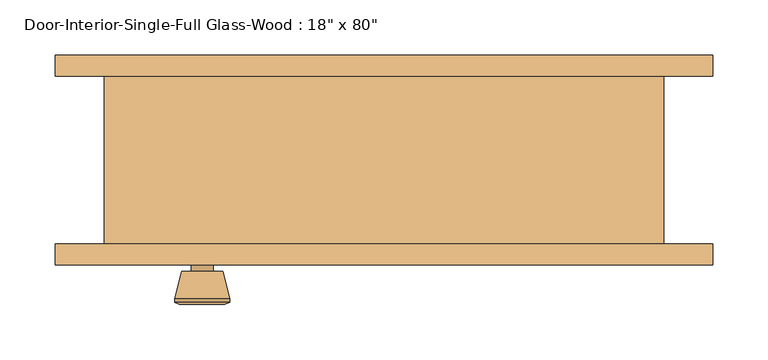
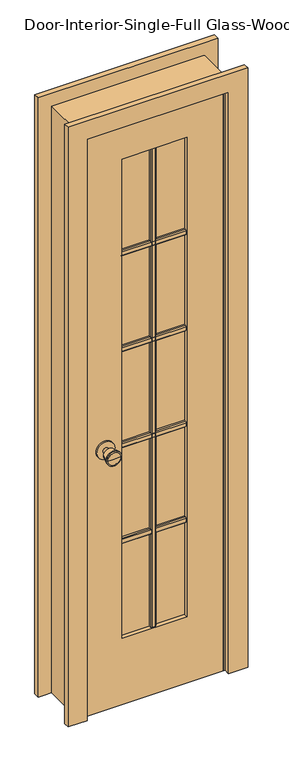
"""IFC4 building model written with IfcOpenShell, lengths in millimetres: door geometry."""

from ifc_helpers import new_model, si_unit, point, frame, frame_2d, origin, place, context, project, spatial, polyline, circle_curve, trimmed, segment, composite_curve, outline, extrude, faceted_brep, source, transform, mapped, element, save
from ifc_brep_helpers import plane_surface, cylinder_surface, revolved_surface, advanced_brep


def door_059bf842(model_context):
    return source(origin(), model_context, "Body", "SolidModel", [
        extrude(outline(polyline([(-59.055, 1586.23), (-59.055, 1567.18), (-65.405, 1567.18), (-68.58, 1570.355), (-68.58, 1583.055), (-65.405, 1586.23), (-59.055, 1586.23)])), frame((-107.95, 0.0, 0.0), z_axis=(1.0, 0.0, 0.0), x_axis=(0.0, 1.0, 0.0)), (0.0, 0.0, 1.0), 215.9),
        extrude(outline(polyline([(-59.055, 1249.9975), (-59.055, 1230.9475), (-65.405, 1230.9475), (-68.58, 1234.1225), (-68.58, 1246.8225), (-65.405, 1249.9975), (-59.055, 1249.9975)])), frame((-107.95, 0.0, 0.0), z_axis=(1.0, 0.0, 0.0), x_axis=(0.0, 1.0, 0.0)), (0.0, 0.0, 1.0), 215.9),
        extrude(outline(polyline([(-59.055, 913.765), (-59.055, 894.715), (-65.405, 894.715), (-68.58, 897.89), (-68.58, 910.59), (-65.405, 913.765), (-59.055, 913.765)])), frame((-107.95, 0.0, 0.0), z_axis=(1.0, 0.0, 0.0), x_axis=(0.0, 1.0, 0.0)), (0.0, 0.0, 1.0), 215.9),
        extrude(outline(polyline([(-9.525, -59.055), (9.525, -59.055), (9.525, -65.405), (6.35, -68.58), (-6.35, -68.58), (-9.525, -65.405), (-9.525, -59.055)])), frame((0.0, 0.0, 231.775), z_axis=(0.0, 0.0, 1.0), x_axis=(1.0, 0.0, 0.0)), (0.0, 0.0, 1.0), 1681.1625),
        extrude(outline(polyline([(-59.055, 577.5325), (-59.055, 558.4825), (-65.405, 558.4825), (-68.58, 561.6575), (-68.58, 574.3575), (-65.405, 577.5325), (-59.055, 577.5325)])), frame((-107.95, 0.0, 0.0), z_axis=(1.0, 0.0, 0.0), x_axis=(0.0, 1.0, 0.0)), (0.0, 0.0, 1.0), 215.9),
        extrude(outline(polyline([(-52.07, 1586.23), (-45.72, 1586.23), (-42.545, 1583.055), (-42.545, 1570.355), (-45.72, 1567.18), (-52.07, 1567.18), (-52.07, 1586.23)])), frame((-107.95, 0.0, 0.0), z_axis=(1.0, 0.0, 0.0), x_axis=(0.0, 1.0, 0.0)), (0.0, 0.0, 1.0), 215.9),
        extrude(outline(polyline([(-52.07, 1249.9975), (-45.72, 1249.9975), (-42.545, 1246.8225), (-42.545, 1234.1225), (-45.72, 1230.9475), (-52.07, 1230.9475), (-52.07, 1249.9975)])), frame((-107.95, 0.0, 0.0), z_axis=(1.0, 0.0, 0.0), x_axis=(0.0, 1.0, 0.0)), (0.0, 0.0, 1.0), 215.9),
        extrude(outline(polyline([(-52.07, 913.765), (-45.72, 913.765), (-42.545, 910.59), (-42.545, 897.89), (-45.72, 894.715), (-52.07, 894.715), (-52.07, 913.765)])), frame((-107.95, 0.0, 0.0), z_axis=(1.0, 0.0, 0.0), x_axis=(0.0, 1.0, 0.0)), (0.0, 0.0, 1.0), 215.9),
        extrude(outline(polyline([(-9.525, -52.07), (-9.525, -45.72), (-6.35, -42.545), (6.35, -42.545), (9.525, -45.72), (9.525, -52.07), (-9.525, -52.07)])), frame((0.0, 0.0, 231.775), z_axis=(0.0, 0.0, 1.0), x_axis=(1.0, 0.0, 0.0)), (0.0, 0.0, 1.0), 1681.1625),
        extrude(outline(polyline([(-52.07, 577.5325), (-45.72, 577.5325), (-42.545, 574.3575), (-42.545, 561.6575), (-45.72, 558.4825), (-52.07, 558.4825), (-52.07, 577.5325)])), frame((-107.95, 0.0, 0.0), z_axis=(1.0, 0.0, 0.0), x_axis=(0.0, 1.0, 0.0)), (0.0, 0.0, 1.0), 215.9),
        advanced_brep(
        [(-165.1, -32.1, 914.4), (-175.1, -32.1, 914.4), (-155.1, -32.1, 914.4), (-144.6241324, 16.9, 914.4), (-185.5758676, 16.9, 914.4), (-165.1, 16.9, 914.4), (-140.1, 15.0721319, 914.4), (-190.1, 15.0721319, 914.4), (-140.1, 11.6084537, 914.4), (-190.1, 11.6084537, 914.4), (-146.463764, -13.1, 914.4), (-183.736236, -13.1, 914.4), (-155.1, -13.1, 914.4), (-175.1, -13.1, 914.4)],
        [
            (0, 1),
            (1, 2, circle_curve(frame((-165.1, -32.1, 914.4), z_axis=(0.0, -1.0, 0.0), x_axis=(-1.0, 0.0, 0.0)), 10.0)),
            (2, 0),
            (2, 1, circle_curve(frame((-165.1, -32.1, 914.4), z_axis=(0.0, -1.0, 0.0), x_axis=(-1.0, 0.0, 0.0)), 10.0)),
            (3, 4, circle_curve(frame((-165.1, 16.9, 914.4), z_axis=(0.0, 1.0, 0.0), x_axis=(-1.0, 0.0, 0.0)), 20.4758676)),
            (4, 5),
            (5, 3),
            (4, 3, circle_curve(frame((-165.1, 16.9, 914.4), z_axis=(0.0, 1.0, 0.0), x_axis=(-1.0, 0.0, 0.0)), 20.4758676)),
            (6, 7, circle_curve(frame((-165.1, 15.0721319, 914.4), z_axis=(0.0, 1.0, 0.0), x_axis=(-1.0, 0.0, 0.0)), 25.0)),
            (7, 4),
            (3, 6),
            (7, 6, circle_curve(frame((-165.1, 15.0721319, 914.4), z_axis=(0.0, 1.0, 0.0), x_axis=(-1.0, 0.0, 0.0)), 25.0)),
            (8, 9, circle_curve(frame((-165.1, 11.6084537, 914.4), z_axis=(0.0, 1.0, 0.0), x_axis=(-1.0, 0.0, 0.0)), 25.0)),
            (9, 7),
            (6, 8),
            (9, 8, circle_curve(frame((-165.1, 11.6084537, 914.4), z_axis=(0.0, 1.0, 0.0), x_axis=(-1.0, 0.0, 0.0)), 25.0)),
            (10, 11, circle_curve(frame((-165.1, -13.1, 914.4), z_axis=(0.0, 1.0, 0.0), x_axis=(-1.0, 0.0, 0.0)), 18.636236)),
            (11, 9),
            (8, 10),
            (11, 10, circle_curve(frame((-165.1, -13.1, 914.4), z_axis=(0.0, 1.0, 0.0), x_axis=(-1.0, 0.0, 0.0)), 18.636236)),
            (12, 13, circle_curve(frame((-165.1, -13.1, 914.4), z_axis=(0.0, 1.0, 0.0), x_axis=(-1.0, 0.0, 0.0)), 10.0)),
            (13, 11),
            (10, 12),
            (13, 12, circle_curve(frame((-165.1, -13.1, 914.4), z_axis=(0.0, 1.0, 0.0), x_axis=(-1.0, 0.0, 0.0)), 10.0)),
            (1, 13),
            (12, 2),
        ],
        [
            plane_surface(frame((-165.1, -32.1, 914.4), z_axis=(0.0, -1.0, 0.0), x_axis=(-1.0, 0.0, 0.0))),
            plane_surface(frame((-165.1, 16.9, 914.4), z_axis=(0.0, 1.0, 0.0), x_axis=(-1.0, 0.0, 0.0))),
            revolved_surface(polyline([(-185.5758676, 16.9, 914.4), (-190.1, 15.0721319, 914.4)]), (-165.1, -32.1, 914.4), (0.0, -1.0, 0.0)),
            cylinder_surface(frame((-165.1, -32.1, 914.4), z_axis=(0.0, -1.0, 0.0), x_axis=(-1.0, 0.0, 0.0)), 25.0),
            revolved_surface(polyline([(-190.1, 11.6084537, 914.4), (-183.736236, -13.1, 914.4)]), (-165.1, -32.1, 914.4), (0.0, -1.0, 0.0)),
            plane_surface(frame((-165.1, -13.1, 914.4), z_axis=(0.0, -1.0, 0.0), x_axis=(-1.0, 0.0, 0.0))),
            cylinder_surface(frame((-165.1, -32.1, 914.4), z_axis=(0.0, -1.0, 0.0), x_axis=(-1.0, 0.0, 0.0)), 10.0),
        ],
        [
            (0, [[1, 2, 3]]),
            (0, [[-3, 4, -1]]),
            (1, [[5, 6, 7]]),
            (1, [[8, -7, -6]]),
            (2, [[9, 10, -5, 11]]),
            (2, [[12, -11, -8, -10]]),
            (3, [[13, 14, -9, 15]]),
            (3, [[16, -15, -12, -14]]),
            (4, [[17, 18, -13, 19]]),
            (4, [[20, -19, -16, -18]]),
            (5, [[21, 22, -17, 23]]),
            (5, [[24, -23, -20, -22]]),
            (6, [[-2, 25, -21, 26]]),
            (6, [[-4, -26, -24, -25]]),
        ],
    ),
        extrude(outline(composite_curve([segment(trimmed(circle_curve(frame_2d((914.4, -165.1)), 30.0), [point((914.4, -195.1))], [point((914.4, -135.1))], False, "CARTESIAN"), True, "CONTINUOUS"), segment(trimmed(circle_curve(frame_2d((914.4, -165.1)), 30.0), [point((914.4, -135.1))], [point((914.4, -195.1))], False, "CARTESIAN"), True, "CONTINUOUS")], self_intersect=False)), frame((0.0, -38.1, 0.0), z_axis=(0.0, 1.0, 0.0), x_axis=(0.0, 0.0, 1.0)), (0.0, 0.0, 1.0), 6.0),
        advanced_brep(
        [(-165.1, -79.025, 914.4), (-155.1, -79.025, 914.4), (-175.1, -79.025, 914.4), (-144.6241324, -128.025, 914.4), (-165.1, -128.025, 914.4), (-185.5758676, -128.025, 914.4), (-140.1, -126.1971319, 914.4), (-190.1, -126.1971319, 914.4), (-140.1, -122.7334537, 914.4), (-190.1, -122.7334537, 914.4), (-146.463764, -98.025, 914.4), (-183.736236, -98.025, 914.4), (-155.1, -98.025, 914.4), (-175.1, -98.025, 914.4)],
        [
            (0, 1),
            (1, 2, circle_curve(frame((-165.1, -79.025, 914.4), z_axis=(0.0, 1.0, 0.0), x_axis=(-1.0, 0.0, 0.0)), 10.0)),
            (2, 0),
            (2, 1, circle_curve(frame((-165.1, -79.025, 914.4), z_axis=(0.0, 1.0, 0.0), x_axis=(-1.0, 0.0, 0.0)), 10.0)),
            (3, 4),
            (4, 5),
            (5, 3, circle_curve(frame((-165.1, -128.025, 914.4), z_axis=(0.0, -1.0, 0.0), x_axis=(-1.0, 0.0, 0.0)), 20.4758676)),
            (3, 5, circle_curve(frame((-165.1, -128.025, 914.4), z_axis=(0.0, -1.0, 0.0), x_axis=(-1.0, 0.0, 0.0)), 20.4758676)),
            (6, 3),
            (5, 7),
            (7, 6, circle_curve(frame((-165.1, -126.1971319, 914.4), z_axis=(0.0, -1.0, 0.0), x_axis=(-1.0, 0.0, 0.0)), 25.0)),
            (6, 7, circle_curve(frame((-165.1, -126.1971319, 914.4), z_axis=(0.0, -1.0, 0.0), x_axis=(-1.0, 0.0, 0.0)), 25.0)),
            (8, 6),
            (7, 9),
            (9, 8, circle_curve(frame((-165.1, -122.7334537, 914.4), z_axis=(0.0, -1.0, 0.0), x_axis=(-1.0, 0.0, 0.0)), 25.0)),
            (8, 9, circle_curve(frame((-165.1, -122.7334537, 914.4), z_axis=(0.0, -1.0, 0.0), x_axis=(-1.0, 0.0, 0.0)), 25.0)),
            (10, 8),
            (9, 11),
            (11, 10, circle_curve(frame((-165.1, -98.025, 914.4), z_axis=(0.0, -1.0, 0.0), x_axis=(-1.0, 0.0, 0.0)), 18.636236)),
            (10, 11, circle_curve(frame((-165.1, -98.025, 914.4), z_axis=(0.0, -1.0, 0.0), x_axis=(-1.0, 0.0, 0.0)), 18.636236)),
            (12, 10),
            (11, 13),
            (13, 12, circle_curve(frame((-165.1, -98.025, 914.4), z_axis=(0.0, -1.0, 0.0), x_axis=(-1.0, 0.0, 0.0)), 10.0)),
            (12, 13, circle_curve(frame((-165.1, -98.025, 914.4), z_axis=(0.0, -1.0, 0.0), x_axis=(-1.0, 0.0, 0.0)), 10.0)),
            (1, 12),
            (13, 2),
        ],
        [
            plane_surface(frame((-165.1, -79.025, 914.4), z_axis=(0.0, 1.0, 0.0), x_axis=(-1.0, 0.0, 0.0))),
            plane_surface(frame((-165.1, -128.025, 914.4), z_axis=(0.0, -1.0, 0.0), x_axis=(-1.0, 0.0, 0.0))),
            revolved_surface(polyline([(-185.5758676, -128.025, 914.4), (-190.1, -126.1971319, 914.4)]), (-165.1, -79.025, 914.4), (0.0, 1.0, 0.0)),
            cylinder_surface(frame((-165.1, -79.025, 914.4), z_axis=(0.0, 1.0, 0.0), x_axis=(-1.0, 0.0, 0.0)), 25.0),
            revolved_surface(polyline([(-190.1, -122.7334537, 914.4), (-183.736236, -98.025, 914.4)]), (-165.1, -79.025, 914.4), (0.0, 1.0, 0.0)),
            plane_surface(frame((-165.1, -98.025, 914.4), z_axis=(0.0, 1.0, 0.0), x_axis=(-1.0, 0.0, 0.0))),
            cylinder_surface(frame((-165.1, -79.025, 914.4), z_axis=(0.0, 1.0, 0.0), x_axis=(-1.0, 0.0, 0.0)), 10.0),
        ],
        [
            (0, [[1, 2, 3]]),
            (0, [[-3, 4, -1]]),
            (1, [[5, 6, 7]]),
            (1, [[-6, -5, 8]]),
            (2, [[9, -7, 10, 11]]),
            (2, [[-10, -8, -9, 12]]),
            (3, [[13, -11, 14, 15]]),
            (3, [[-14, -12, -13, 16]]),
            (4, [[17, -15, 18, 19]]),
            (4, [[-18, -16, -17, 20]]),
            (5, [[21, -19, 22, 23]]),
            (5, [[-22, -20, -21, 24]]),
            (6, [[25, -23, 26, -2]]),
            (6, [[-26, -24, -25, -4]]),
        ],
    ),
        extrude(outline(composite_curve([segment(trimmed(circle_curve(frame_2d((914.4, -165.1)), 30.0), [point((914.4, -195.1))], [point((914.4, -135.1))], False, "CARTESIAN"), True, "CONTINUOUS"), segment(trimmed(circle_curve(frame_2d((914.4, -165.1)), 30.0), [point((914.4, -135.1))], [point((914.4, -195.1))], False, "CARTESIAN"), True, "CONTINUOUS")], self_intersect=False)), frame((0.0, -79.025, 0.0), z_axis=(0.0, 1.0, 0.0), x_axis=(0.0, 0.0, 1.0)), (0.0, 0.0, 1.0), 6.0),
        extrude(outline(polyline([(2032.0, -228.6), (0.0, -228.6), (0.0, 228.6), (2032.0, 228.6), (2032.0, -228.6)]), holes=[polyline([(1912.9375, -107.95), (1912.9375, 107.95), (231.775, 107.95), (231.775, -107.95), (1912.9375, -107.95)])]), frame((0.0, -73.025, 0.0), z_axis=(0.0, 1.0, 0.0), x_axis=(0.0, 0.0, 1.0)), (0.0, 0.0, 1.0), 34.925),
        faceted_brep([(254.0, -73.025, 0.0), (228.6, -73.025, 0.0), (228.6, -38.1, 0.0), (215.9, -38.1, 0.0), (215.9, -3.175, 0.0), (228.6, -3.175, 0.0), (228.6, 79.375, 0.0), (254.0, 79.375, 0.0), (254.0, 79.375, 2057.4), (254.0, -73.025, 2057.4), (228.6, 79.375, 2032.0), (-228.6, 79.375, 2032.0), (-228.6, 79.375, 0.0), (-254.0, 79.375, 0.0), (-254.0, 79.375, 2057.4), (228.6, -3.175, 2032.0), (215.9, -3.175, 2019.3), (-215.9, -3.175, 2019.3), (-215.9, -3.175, 0.0), (-228.6, -3.175, 0.0), (-228.6, -3.175, 2032.0), (215.9, -38.1, 2019.3), (228.6, -38.1, 2032.0), (-228.6, -38.1, 2032.0), (-228.6, -38.1, 0.0), (-215.9, -38.1, 0.0), (-215.9, -38.1, 2019.3), (228.6, -73.025, 2032.0), (-254.0, -73.025, 2057.4), (-254.0, -73.025, 0.0), (-228.6, -73.025, 0.0), (-228.6, -73.025, 2032.0)], [[[0, 1, 2, 3, 4, 5, 6, 7]], [[7, 8, 9, 0]], [[6, 10, 11, 12, 13, 14, 8, 7]], [[5, 15, 10, 6]], [[4, 16, 17, 18, 19, 20, 15, 5]], [[3, 21, 16, 4]], [[2, 22, 23, 24, 25, 26, 21, 3]], [[1, 27, 22, 2]], [[0, 9, 28, 29, 30, 31, 27, 1]], [[8, 14, 28, 9]], [[15, 20, 11, 10]], [[21, 26, 17, 16]], [[27, 31, 23, 22]], [[29, 13, 12, 19, 18, 25, 24, 30]], [[14, 13, 29, 28]], [[20, 19, 12, 11]], [[26, 25, 18, 17]], [[31, 30, 24, 23]]]),
        extrude(outline(polyline([(107.95, -52.07), (107.95, -59.055), (-107.95, -59.055), (-107.95, -52.07), (107.95, -52.07)])), frame((0.0, 0.0, 231.775), z_axis=(0.0, 0.0, 1.0), x_axis=(1.0, 0.0, 0.0)), (0.0, 0.0, 1.0), 1681.1625),
        extrude(outline(polyline([(0.0, 298.45), (2101.85, 298.45), (2101.85, -298.45), (0.0, -298.45), (0.0, -234.95), (2038.35, -234.95), (2038.35, 234.95), (0.0, 234.95), (0.0, 298.45)])), frame((0.0, 79.375, 0.0), z_axis=(0.0, 1.0, 0.0), x_axis=(0.0, 0.0, 1.0)), (0.0, 0.0, 1.0), 19.05),
        extrude(outline(polyline([(0.0, 298.45), (2101.85, 298.45), (2101.85, -298.45), (0.0, -298.45), (0.0, -234.95), (2038.35, -234.95), (2038.35, 234.95), (0.0, 234.95), (0.0, 298.45)])), frame((0.0, -92.075, 0.0), z_axis=(0.0, 1.0, 0.0), x_axis=(0.0, 0.0, 1.0)), (0.0, 0.0, 1.0), 19.05),
    ])


if __name__ == "__main__":
    model = new_model("IFC4")
    model_context = context("Model", 3, world=origin())
    ifc_project = project(units=[si_unit("LENGTHUNIT", "METRE", prefix="MILLI")], contexts=[model_context])
    site = spatial("IfcSite", under=ifc_project)
    building = spatial("IfcBuilding", under=site)
    placement = place(None, origin())
    door_shape = door_059bf842(model_context)
    element("IfcDoor", 1, ObjectType="Door-Interior-Single-Full Glass-Wood : 18\" x 80\"", at=placement, inside=building, context=model_context, shape_type="MappedRepresentation", body=[
        mapped(door_shape, transform((0.0, 0.0, 0.0), x_axis=(1.0, 0.0, 0.0), y_axis=(0.0, 1.0, 0.0), z_axis=(0.0, 0.0, 1.0))),
    ])
    save(model, "model.ifc")

# Revit data of these elements
# Type "Door-Interior-Single-Full Glass-Wood : 18\" x 80\""
#   Type Mark = "10"
#   Assembly Code = "C1020300"
#   Analytic Construction = "Wood frame with single clear glass"
#   Top Rail = 0' - 4 11/16"
#   Thickness = 0' - 1 3/8"
#   Thermal Resistance (R) = 1.0102 (h·ft²·°F)/BTU
#   Swing Angle [instance default] = 90.00°
#   Stiles = 0' - 4 3/4"
#   Rough Width = 1' - 8"
#   Rough Height = 6' - 9"
#   Height = 6' - 8"
#   Width = 1' - 6"
#   Heat Transfer Coefficient (U) = 0.9900 BTU/(h·ft²·°F)
#   Bottom Rail = 0' - 9 1/8"
#   Show Grill [instance default] = yes
#   Trim Material = Cherry
#   Panel Material = Cherry
#   Frame Material = Cherry
#   Door Handle Material = Aluminum
#   Visual Light Transmittance = 0
#   Solar Heat Gain Coefficient = 0
#   Wall Closure = (empty or 0)
#   Function = (empty or 0)
# Element 1 (IfcDoor, "Door-Interior-Single-Full Glass-Wood : 18\" x 80\"")
#   Materials on its faces: "Cherry", "Aluminum", "Glass"
# Materials
#   "Cherry": class "Wood", colour RGB 226 177 128, transparency 0, Description = "Prunus Serotina", Cost = 0
#   "Aluminum": class "Metal", colour RGB 247 247 247, transparency 0, Description = "Aluminum 6061", Cost = 0
#   "Glass": class "Glass", colour RGB 0 128 192, transparency 0.75, Description = "Soda Lime Glass", Cost = 0
